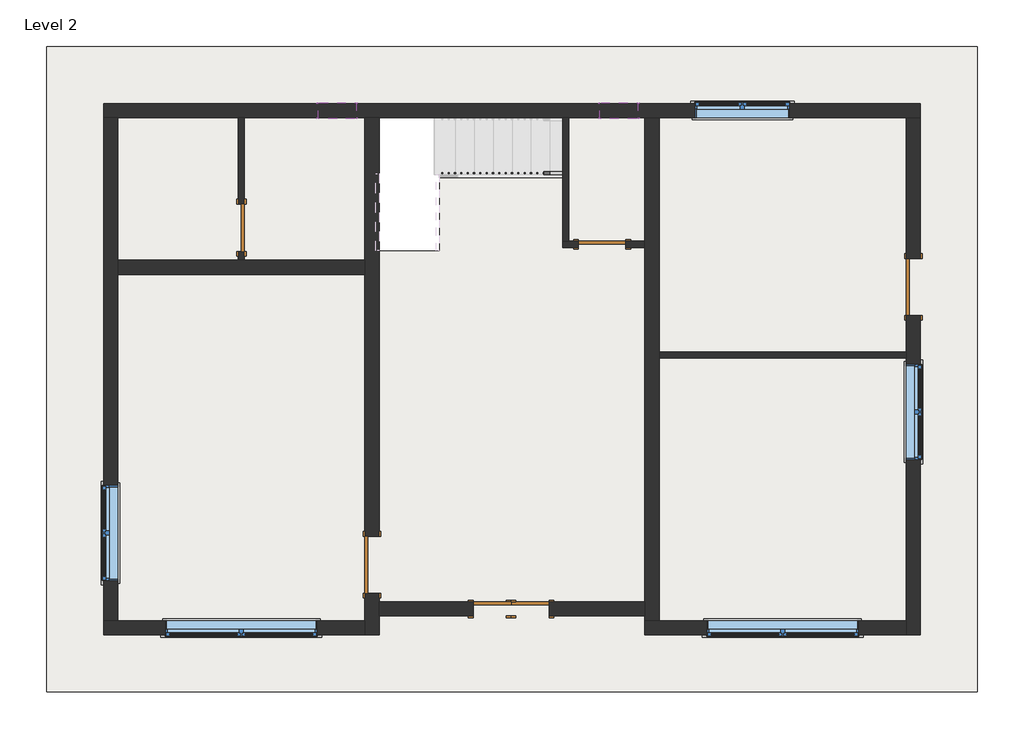
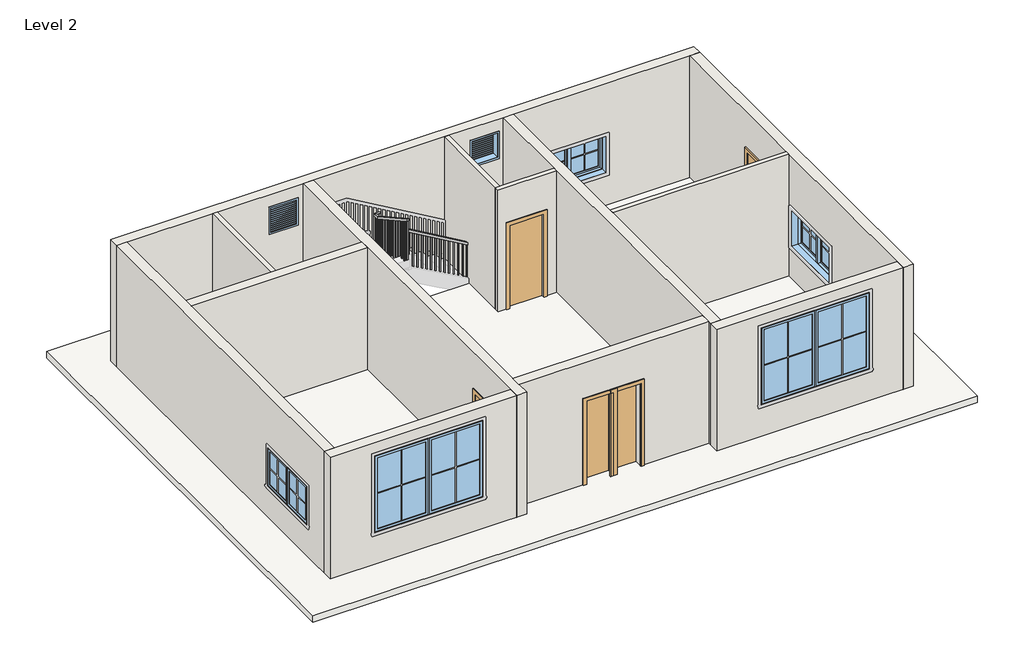
# One storey, part 1 of 2: 13 walls, 7 windows, 6 doors, 1 railing, 1 roof.
"""IFC4 building model written with IfcOpenShell, lengths in millimetres."""

from ifc_helpers import new_model, si_unit, frame, origin, place, context, project, spatial, polyline, outline, extrude, faceted_brep, transform, mapped, element, save
from components import single_flush_door_2_4a3212df, single_flush_door_2_0d3b4037, door_270f2424, door_aa9e95e7, single_flush_door_3_a90ba1ad, window_casement_double_c1d95f0f, window_casement_double_9ae172a2, window_f2d8fef0

model = new_model("IFC4")

# Units and contexts
model_context = context("Model", 3, world=origin())
ifc_project = project(units=[si_unit("LENGTHUNIT", "METRE", prefix="MILLI")], contexts=[model_context])

# Site, building, storey
site = spatial("IfcSite", under=ifc_project)
building = spatial("IfcBuilding", under=site)
storey = spatial("IfcBuildingStorey", under=building, Name="Level 2", Elevation=3048.0)

# Doors
placement = place(None, origin())
single_flush_door_2_shape = single_flush_door_2_4a3212df(model_context)
element("IfcDoor", 1, ObjectType="Single-Flush : DOOR 2'", at=placement, inside=storey, context=model_context, shape_type="MappedRepresentation", body=[
    mapped(single_flush_door_2_shape, transform((-1572.7415084, -2604.3618005, 3048.0), x_axis=(-1.0, 0.0, 0.0), y_axis=(0.0, -1.0, 0.0), z_axis=(0.0, 0.0, 1.0))),
])
single_flush_door_2_2_shape = single_flush_door_2_0d3b4037(model_context)
element("IfcDoor", 2, ObjectType="Single-Flush : DOOR 2'", at=placement, inside=storey, context=model_context, shape_type="MappedRepresentation", body=[
    mapped(single_flush_door_2_2_shape, transform((-963.1415084, -2604.3618005, 3048.0), x_axis=(1.0, 0.0, 0.0), y_axis=(0.0, 1.0, 0.0), z_axis=(0.0, 0.0, 1.0))),
])
door_shape = door_270f2424(model_context)
element("IfcDoor", 3, ObjectType="Single-Flush : DOOR 2'6\"", at=placement, inside=storey, context=model_context, shape_type="MappedRepresentation", body=[
    mapped(door_shape, transform((-5598.6415084, 3517.0381995, 3048.0), x_axis=(0.0, -1.0, 0.0), y_axis=(1.0, 0.0, 0.0), z_axis=(0.0, 0.0, 1.0))),
])
door_2_shape = door_aa9e95e7(model_context)
element("IfcDoor", 4, ObjectType="Single-Flush : DOOR 2'6\"", at=placement, inside=storey, context=model_context, shape_type="MappedRepresentation", body=[
    mapped(door_2_shape, transform((192.5584916, 3250.3381995, 3048.0), x_axis=(-1.0, 0.0, 0.0), y_axis=(0.0, -1.0, 0.0), z_axis=(0.0, 0.0, 1.0))),
])
single_flush_door_3_shape = single_flush_door_3_a90ba1ad(model_context)
element("IfcDoor", 5, ObjectType="Single-Flush : DOOR 3'", at=placement, inside=storey, context=model_context, shape_type="MappedRepresentation", body=[
    mapped(single_flush_door_3_shape, transform((-3503.1415084, -1893.1618005, 3048.0), x_axis=(0.0, -1.0, 0.0), y_axis=(1.0, 0.0, 0.0), z_axis=(0.0, 0.0, 1.0))),
])
element("IfcDoor", 6, ObjectType="Single-Flush : DOOR 3'", at=placement, inside=storey, context=model_context, shape_type="MappedRepresentation", body=[
    mapped(single_flush_door_3_shape, transform((5183.6584916, 2564.5381995, 3048.0), x_axis=(0.0, -1.0, 0.0), y_axis=(1.0, 0.0, 0.0), z_axis=(0.0, 0.0, 1.0))),
])

# Railing
element("IfcRailing", 7, ObjectType="Handrail - Rectangular", at=placement, inside=storey, context=model_context, shape_type="SolidModel", body=[
    faceted_brep([(-442.4415084, 4368.3146777, 4131.7333333), (-442.4415084, 4368.3146777, 4072.9219871), (-442.4415084, 4419.1146777, 4072.9219871), (-442.4415084, 4419.1146777, 4131.7333333), (-2398.2415084, 4368.3146777, 5272.6166667), (-2449.0415084, 4368.3146777, 5243.4386538), (-2449.0415084, 4419.1146777, 5243.4386538), (-2398.2415084, 4419.1146777, 5272.6166667), (-2398.2415084, 4368.3146777, 5528.7202697), (-2449.0415084, 4368.3146777, 5477.9202697), (-2449.0415084, 4419.1146777, 5477.9202697), (-2398.2415084, 4419.1146777, 5528.7202697), (-2474.4415084, 4368.3146777, 5528.7202697), (-2474.4415084, 4368.3146777, 5477.9202697), (-2525.2415084, 4419.1146777, 5477.9202697), (-2525.2415084, 4419.1146777, 5528.7202697), (-2474.4415084, 4292.1146777, 5528.7202697), (-2474.4415084, 4278.9546266, 5477.9202697), (-2525.2415084, 4278.9546266, 5477.9202697), (-2525.2415084, 4292.1146777, 5528.7202697), (-2474.4415084, 3148.7383287, 6163.7333333), (-2525.2415084, 3148.7383287, 6163.7333333), (-2525.2415084, 3148.7383287, 6105.62445), (-2474.4415084, 3148.7383287, 6105.62445)], [[[0, 1, 2, 3]], [[1, 0, 4, 5]], [[2, 1, 5, 6]], [[3, 2, 6, 7]], [[0, 3, 7, 4]], [[5, 4, 8, 9]], [[6, 5, 9, 10]], [[7, 6, 10, 11]], [[4, 7, 11, 8]], [[9, 8, 12, 13]], [[10, 9, 13, 14]], [[11, 10, 14, 15]], [[8, 11, 15, 12]], [[13, 12, 16, 17]], [[14, 13, 17, 18]], [[15, 14, 18, 19]], [[12, 15, 19, 16]], [[20, 21, 22, 23]], [[17, 16, 20, 23]], [[18, 17, 23, 22]], [[19, 18, 22, 21]], [[16, 19, 21, 20]]]),
    extrude(outline(polyline([(3184.0396777, 6086.1754052), (3184.0396777, 5080.0), (3164.9896777, 5080.0), (3164.9896777, 6096.7554726), (3184.0396777, 6086.1754052)])), frame((-2509.3665084, 0.0, 0.0), z_axis=(1.0, 0.0, 0.0), x_axis=(0.0, 1.0, 0.0)), (0.0, 0.0, 1.0), 19.05),
    extrude(outline(polyline([(3285.6396777, 6029.7483789), (3285.6396777, 5080.0), (3266.5896777, 5080.0), (3266.5896777, 6040.3284463), (3285.6396777, 6029.7483789)])), frame((-2509.3665084, 0.0, 0.0), z_axis=(1.0, 0.0, 0.0), x_axis=(0.0, 1.0, 0.0)), (0.0, 0.0, 1.0), 19.05),
    extrude(outline(polyline([(3387.2396777, 5973.3213526), (3387.2396777, 5080.0), (3368.1896777, 5080.0), (3368.1896777, 5983.9014201), (3387.2396777, 5973.3213526)])), frame((-2509.3665084, 0.0, 0.0), z_axis=(1.0, 0.0, 0.0), x_axis=(0.0, 1.0, 0.0)), (0.0, 0.0, 1.0), 19.05),
    extrude(outline(polyline([(3488.8396777, 5916.8420718), (3488.8396777, 4910.6666667), (3469.7896777, 4910.6666667), (3469.7896777, 5927.4221392), (3488.8396777, 5916.8420718)])), frame((-2509.3665084, 0.0, 0.0), z_axis=(1.0, 0.0, 0.0), x_axis=(0.0, 1.0, 0.0)), (0.0, 0.0, 1.0), 19.05),
    extrude(outline(polyline([(3590.4396777, 5860.4150456), (3590.4396777, 4910.6666667), (3571.3896777, 4910.6666667), (3571.3896777, 5870.995113), (3590.4396777, 5860.4150456)])), frame((-2509.3665084, 0.0, 0.0), z_axis=(1.0, 0.0, 0.0), x_axis=(0.0, 1.0, 0.0)), (0.0, 0.0, 1.0), 19.05),
    extrude(outline(polyline([(3692.0396777, 5803.9880193), (3692.0396777, 4910.6666667), (3672.9896777, 4910.6666667), (3672.9896777, 5814.5680867), (3692.0396777, 5803.9880193)])), frame((-2509.3665084, 0.0, 0.0), z_axis=(1.0, 0.0, 0.0), x_axis=(0.0, 1.0, 0.0)), (0.0, 0.0, 1.0), 19.05),
    extrude(outline(polyline([(3793.6396777, 5747.5087385), (3793.6396777, 4741.3333333), (3774.5896777, 4741.3333333), (3774.5896777, 5758.0888059), (3793.6396777, 5747.5087385)])), frame((-2509.3665084, 0.0, 0.0), z_axis=(1.0, 0.0, 0.0), x_axis=(0.0, 1.0, 0.0)), (0.0, 0.0, 1.0), 19.05),
    extrude(outline(polyline([(3895.2396777, 5691.0817122), (3895.2396777, 4741.3333333), (3876.1896777, 4741.3333333), (3876.1896777, 5701.6617797), (3895.2396777, 5691.0817122)])), frame((-2509.3665084, 0.0, 0.0), z_axis=(1.0, 0.0, 0.0), x_axis=(0.0, 1.0, 0.0)), (0.0, 0.0, 1.0), 19.05),
    extrude(outline(polyline([(3996.8396777, 5634.654686), (3996.8396777, 4741.3333333), (3977.7896777, 4741.3333333), (3977.7896777, 5645.2347534), (3996.8396777, 5634.654686)])), frame((-2509.3665084, 0.0, 0.0), z_axis=(1.0, 0.0, 0.0), x_axis=(0.0, 1.0, 0.0)), (0.0, 0.0, 1.0), 19.05),
    extrude(outline(polyline([(4098.4396777, 5578.1754052), (4098.4396777, 4572.0), (4079.3896777, 4572.0), (4079.3896777, 5588.7554726), (4098.4396777, 5578.1754052)])), frame((-2509.3665084, 0.0, 0.0), z_axis=(1.0, 0.0, 0.0), x_axis=(0.0, 1.0, 0.0)), (0.0, 0.0, 1.0), 19.05),
    extrude(outline(polyline([(4200.0396777, 5521.7483789), (4200.0396777, 4572.0), (4180.9896777, 4572.0), (4180.9896777, 5532.3284463), (4200.0396777, 5521.7483789)])), frame((-2509.3665084, 0.0, 0.0), z_axis=(1.0, 0.0, 0.0), x_axis=(0.0, 1.0, 0.0)), (0.0, 0.0, 1.0), 19.05),
    extrude(outline(polyline([(4301.6396777, 5465.3213526), (4301.6396777, 4572.0), (4282.5896777, 4572.0), (4282.5896777, 5475.9014201), (4301.6396777, 5465.3213526)])), frame((-2509.3665084, 0.0, 0.0), z_axis=(1.0, 0.0, 0.0), x_axis=(0.0, 1.0, 0.0)), (0.0, 0.0, 1.0), 19.05),
    extrude(outline(polyline([(-2464.9165084, 4384.1896777), (-2483.9665084, 4384.1896777), (-2483.9665084, 4403.2396777), (-2464.9165084, 4403.2396777), (-2464.9165084, 4384.1896777)])), frame((0.0, 0.0, 4402.6666667), z_axis=(0.0, 0.0, 1.0), x_axis=(1.0, 0.0, 0.0)), (0.0, 0.0, 1.0), 1075.253603),
    extrude(outline(polyline([(5204.5449038, -2382.3665084), (4233.3333333, -2382.3665084), (4233.3333333, -2363.3165084), (5193.4324038, -2363.3165084), (5204.5449038, -2382.3665084)])), frame((0.0, 4384.1896777, 0.0), z_axis=(0.0, 1.0, 0.0), x_axis=(0.0, 0.0, 1.0)), (0.0, 0.0, 1.0), 19.05),
    extrude(outline(polyline([(5145.2782371, -2280.7665084), (4233.3333333, -2280.7665084), (4233.3333333, -2261.7165084), (5134.1657371, -2261.7165084), (5145.2782371, -2280.7665084)])), frame((0.0, 4384.1896777, 0.0), z_axis=(0.0, 1.0, 0.0), x_axis=(0.0, 0.0, 1.0)), (0.0, 0.0, 1.0), 19.05),
    extrude(outline(polyline([(5086.0115704, -2179.1665084), (4233.3333333, -2179.1665084), (4233.3333333, -2160.1165084), (5074.8990704, -2160.1165084), (5086.0115704, -2179.1665084)])), frame((0.0, 4384.1896777, 0.0), z_axis=(0.0, 1.0, 0.0), x_axis=(0.0, 0.0, 1.0)), (0.0, 0.0, 1.0), 19.05),
    extrude(outline(polyline([(5026.7449038, -2077.5665084), (4064.0, -2077.5665084), (4064.0, -2058.5165084), (5015.6324038, -2058.5165084), (5026.7449038, -2077.5665084)])), frame((0.0, 4384.1896777, 0.0), z_axis=(0.0, 1.0, 0.0), x_axis=(0.0, 0.0, 1.0)), (0.0, 0.0, 1.0), 19.05),
    extrude(outline(polyline([(4967.4782371, -1975.9665084), (4064.0, -1975.9665084), (4064.0, -1956.9165084), (4956.3657371, -1956.9165084), (4967.4782371, -1975.9665084)])), frame((0.0, 4384.1896777, 0.0), z_axis=(0.0, 1.0, 0.0), x_axis=(0.0, 0.0, 1.0)), (0.0, 0.0, 1.0), 19.05),
    extrude(outline(polyline([(4908.2115704, -1874.3665084), (4064.0, -1874.3665084), (4064.0, -1855.3165084), (4897.0990704, -1855.3165084), (4908.2115704, -1874.3665084)])), frame((0.0, 4384.1896777, 0.0), z_axis=(0.0, 1.0, 0.0), x_axis=(0.0, 0.0, 1.0)), (0.0, 0.0, 1.0), 19.05),
    extrude(outline(polyline([(4848.9449038, -1772.7665084), (3894.6666667, -1772.7665084), (3894.6666667, -1753.7165084), (4837.8324038, -1753.7165084), (4848.9449038, -1772.7665084)])), frame((0.0, 4384.1896777, 0.0), z_axis=(0.0, 1.0, 0.0), x_axis=(0.0, 0.0, 1.0)), (0.0, 0.0, 1.0), 19.05),
    extrude(outline(polyline([(4789.6782371, -1671.1665084), (3894.6666667, -1671.1665084), (3894.6666667, -1652.1165084), (4778.5657371, -1652.1165084), (4789.6782371, -1671.1665084)])), frame((0.0, 4384.1896777, 0.0), z_axis=(0.0, 1.0, 0.0), x_axis=(0.0, 0.0, 1.0)), (0.0, 0.0, 1.0), 19.05),
    extrude(outline(polyline([(4730.4115704, -1569.5665084), (3894.6666667, -1569.5665084), (3894.6666667, -1550.5165084), (4719.2990704, -1550.5165084), (4730.4115704, -1569.5665084)])), frame((0.0, 4384.1896777, 0.0), z_axis=(0.0, 1.0, 0.0), x_axis=(0.0, 0.0, 1.0)), (0.0, 0.0, 1.0), 19.05),
    extrude(outline(polyline([(4671.1449038, -1467.9665084), (3725.3333333, -1467.9665084), (3725.3333333, -1448.9165084), (4660.0324038, -1448.9165084), (4671.1449038, -1467.9665084)])), frame((0.0, 4384.1896777, 0.0), z_axis=(0.0, 1.0, 0.0), x_axis=(0.0, 0.0, 1.0)), (0.0, 0.0, 1.0), 19.05),
    extrude(outline(polyline([(4611.8782371, -1366.3665084), (3725.3333333, -1366.3665084), (3725.3333333, -1347.3165084), (4600.7657371, -1347.3165084), (4611.8782371, -1366.3665084)])), frame((0.0, 4384.1896777, 0.0), z_axis=(0.0, 1.0, 0.0), x_axis=(0.0, 0.0, 1.0)), (0.0, 0.0, 1.0), 19.05),
    extrude(outline(polyline([(4552.6115704, -1264.7665084), (3725.3333333, -1264.7665084), (3725.3333333, -1245.7165084), (4541.4990704, -1245.7165084), (4552.6115704, -1264.7665084)])), frame((0.0, 4384.1896777, 0.0), z_axis=(0.0, 1.0, 0.0), x_axis=(0.0, 0.0, 1.0)), (0.0, 0.0, 1.0), 19.05),
    extrude(outline(polyline([(4493.3449038, -1163.1665084), (3556.0, -1163.1665084), (3556.0, -1144.1165084), (4482.2324038, -1144.1165084), (4493.3449038, -1163.1665084)])), frame((0.0, 4384.1896777, 0.0), z_axis=(0.0, 1.0, 0.0), x_axis=(0.0, 0.0, 1.0)), (0.0, 0.0, 1.0), 19.05),
    extrude(outline(polyline([(4434.0782371, -1061.5665084), (3556.0, -1061.5665084), (3556.0, -1042.5165084), (4422.9657371, -1042.5165084), (4434.0782371, -1061.5665084)])), frame((0.0, 4384.1896777, 0.0), z_axis=(0.0, 1.0, 0.0), x_axis=(0.0, 0.0, 1.0)), (0.0, 0.0, 1.0), 19.05),
    extrude(outline(polyline([(4374.8115704, -959.9665084), (3556.0, -959.9665084), (3556.0, -940.9165084), (4363.6990704, -940.9165084), (4374.8115704, -959.9665084)])), frame((0.0, 4384.1896777, 0.0), z_axis=(0.0, 1.0, 0.0), x_axis=(0.0, 0.0, 1.0)), (0.0, 0.0, 1.0), 19.05),
    extrude(outline(polyline([(4315.5449038, -858.3665084), (3386.6666667, -858.3665084), (3386.6666667, -839.3165084), (4304.4324038, -839.3165084), (4315.5449038, -858.3665084)])), frame((0.0, 4384.1896777, 0.0), z_axis=(0.0, 1.0, 0.0), x_axis=(0.0, 0.0, 1.0)), (0.0, 0.0, 1.0), 19.05),
    extrude(outline(polyline([(4256.2782371, -756.7665084), (3386.6666667, -756.7665084), (3386.6666667, -737.7165084), (4245.1657371, -737.7165084), (4256.2782371, -756.7665084)])), frame((0.0, 4384.1896777, 0.0), z_axis=(0.0, 1.0, 0.0), x_axis=(0.0, 0.0, 1.0)), (0.0, 0.0, 1.0), 19.05),
    extrude(outline(polyline([(4197.0115704, -655.1665084), (3386.6666667, -655.1665084), (3386.6666667, -636.1165084), (4185.8990704, -636.1165084), (4197.0115704, -655.1665084)])), frame((0.0, 4384.1896777, 0.0), z_axis=(0.0, 1.0, 0.0), x_axis=(0.0, 0.0, 1.0)), (0.0, 0.0, 1.0), 19.05),
    extrude(outline(polyline([(4137.7449038, -553.5665084), (3217.3333333, -553.5665084), (3217.3333333, -534.5165084), (4126.6324038, -534.5165084), (4137.7449038, -553.5665084)])), frame((0.0, 4384.1896777, 0.0), z_axis=(0.0, 1.0, 0.0), x_axis=(0.0, 0.0, 1.0)), (0.0, 0.0, 1.0), 19.05),
    extrude(outline(polyline([(-2490.3165084, 4384.1896777), (-2509.3665084, 4384.1896777), (-2509.3665084, 4403.2396777), (-2490.3165084, 4403.2396777), (-2490.3165084, 4384.1896777)])), frame((0.0, 0.0, 4402.6666667), z_axis=(0.0, 0.0, 1.0), x_axis=(1.0, 0.0, 0.0)), (0.0, 0.0, 1.0), 1075.253603),
    extrude(outline(polyline([(3167.7883287, 6095.0443826), (3167.7883287, 5080.0), (3148.7383287, 5080.0), (3148.7383287, 6105.62445), (3167.7883287, 6095.0443826)])), frame((-2509.3665084, 0.0, 0.0), z_axis=(1.0, 0.0, 0.0), x_axis=(0.0, 1.0, 0.0)), (0.0, 0.0, 1.0), 19.05),
    extrude(outline(polyline([(4084.0344871, -461.4915084), (3217.3333333, -461.4915084), (3217.3333333, -442.4415084), (4072.9219871, -442.4415084), (4084.0344871, -461.4915084)])), frame((0.0, 4384.1896777, 0.0), z_axis=(0.0, 1.0, 0.0), x_axis=(0.0, 0.0, 1.0)), (0.0, 0.0, 1.0), 19.05),
])

# Roof
element("IfcRoof", 8, ObjectType="ROOF 6\"", at=placement, inside=storey, context=model_context, shape_type="SweptSolid", body=[
    extrude(outline(polyline([(-8722.8415084, -3937.8618005), (-8722.8415084, 6425.3381995), (6212.3584916, 6425.3381995), (6212.3584916, -3937.8618005), (-8722.8415084, -3937.8618005)]), holes=[polyline([(-3439.6415084, 5333.1381995), (-3439.6415084, 3148.7383287), (-2423.6415084, 3148.7383287), (-2423.6415084, 4317.5146777), (-442.4415084, 4317.5146777), (-442.4415084, 5333.1381995), (-3439.6415084, 5333.1381995)])]), frame((0.0, 0.0, 3048.0), z_axis=(0.0, 0.0, 1.0), x_axis=(1.0, 0.0, 0.0)), (0.0, 0.0, 1.0), 152.4),
])

# Walls
element("IfcWall", 9, ObjectType="WALL 4\"", at=placement, inside=storey, context=model_context, shape_type="SweptSolid", body=[
    extrude(outline(polyline([(3136.0381995, 5181.6), (3136.0381995, 3048.0), (2996.3381995, 3048.0), (2996.3381995, 6096.0), (5282.3381995, 6096.0), (5282.3381995, 3048.0), (3898.0381995, 3048.0), (3898.0381995, 5181.6), (3136.0381995, 5181.6)])), frame((-5649.4415084, 0.0, 0.0), z_axis=(1.0, 0.0, 0.0), x_axis=(0.0, 1.0, 0.0)), (0.0, 0.0, 1.0), 101.6),
])
element("IfcWall", 10, ObjectType="WALL 4\"", at=placement, inside=storey, context=model_context, shape_type="Brep", body=[
    faceted_brep([(-188.4415084, 3301.1381995, 5181.6), (-188.4415084, 3301.1381995, 3048.0), (-340.8415084, 3301.1381995, 3048.0), (-442.4415084, 3301.1381995, 3048.0), (-442.4415084, 3301.1381995, 6096.0), (-340.8415084, 3301.1381995, 6096.0), (878.3584916, 3301.1381995, 6096.0), (878.3584916, 3301.1381995, 3048.0), (573.5584916, 3301.1381995, 3048.0), (573.5584916, 3301.1381995, 5181.6), (-442.4415084, 3199.5381995, 3048.0), (-188.4415084, 3199.5381995, 3048.0), (-188.4415084, 3199.5381995, 5181.6), (573.5584916, 3199.5381995, 5181.6), (573.5584916, 3199.5381995, 3048.0), (878.3584916, 3199.5381995, 3048.0), (878.3584916, 3199.5381995, 6096.0), (-442.4415084, 3199.5381995, 6096.0)], [[[0, 1, 2, 3, 4, 5, 6, 7, 8, 9]], [[10, 11, 12, 13, 14, 15, 16, 17]], [[8, 7, 15, 14]], [[3, 2, 1, 11, 10]], [[7, 6, 16, 15]], [[4, 3, 10, 17]], [[12, 11, 1, 0]], [[13, 12, 0, 9]], [[14, 13, 9, 8]], [[6, 5, 4, 17, 16]]]),
])
element("IfcWall", 11, ObjectType="WALL 4\"", at=placement, inside=storey, context=model_context, shape_type="Brep", body=[
    faceted_brep([(-340.8415084, 3301.1381995, 3048.0), (-340.8415084, 5282.3381995, 3048.0), (-340.8415084, 5282.3381995, 6096.0), (-340.8415084, 3301.1381995, 6096.0), (-442.4415084, 3301.1381995, 3048.0), (-442.4415084, 3301.1381995, 6096.0), (-442.4415084, 4317.5146777, 6096.0), (-442.4415084, 5282.3381995, 6096.0), (-442.4415084, 5282.3381995, 3048.0)], [[[0, 1, 2, 3]], [[4, 5, 6, 7, 8]], [[1, 0, 4, 8]], [[0, 3, 5, 4]], [[2, 1, 8, 7]], [[3, 2, 7, 6, 5]]]),
])
element("IfcWall", 12, ObjectType="WALL 4\"", at=placement, inside=storey, context=model_context, shape_type="SweptSolid", body=[
    extrude(outline(polyline([(1106.9584916, 1523.1381995), (5069.3584916, 1523.1381995), (5069.3584916, 1421.5381995), (1106.9584916, 1421.5381995), (1106.9584916, 1523.1381995)])), frame((0.0, 0.0, 3048.0), z_axis=(0.0, 0.0, 1.0), x_axis=(1.0, 0.0, 0.0)), (0.0, 0.0, 1.0), 3048.0),
])
element("IfcWall", 13, ObjectType="WALL 9\"", at=placement, inside=storey, context=model_context, shape_type="Brep", body=[
    faceted_brep([(-7808.4415084, 5282.3381995, 3048.0), (-7579.8415084, 5282.3381995, 3048.0), (-5649.4415084, 5282.3381995, 3048.0), (-5547.8415084, 5282.3381995, 3048.0), (-3617.4415084, 5282.3381995, 3048.0), (-3388.8415084, 5282.3381995, 3048.0), (-442.4415084, 5282.3381995, 3048.0), (-340.8415084, 5282.3381995, 3048.0), (878.3584916, 5282.3381995, 3048.0), (1106.9584916, 5282.3381995, 3048.0), (5069.3584916, 5282.3381995, 3048.0), (5297.9584916, 5282.3381995, 3048.0), (5297.9584916, 5282.3381995, 6096.0), (5069.3584916, 5282.3381995, 6096.0), (1106.9584916, 5282.3381995, 6096.0), (878.3584916, 5282.3381995, 6096.0), (-340.8415084, 5282.3381995, 6096.0), (-442.4415084, 5282.3381995, 6096.0), (-3388.8415084, 5282.3381995, 6096.0), (-3617.4415084, 5282.3381995, 6096.0), (-5547.8415084, 5282.3381995, 6096.0), (-5649.4415084, 5282.3381995, 6096.0), (-7579.8415084, 5282.3381995, 6096.0), (-7808.4415084, 5282.3381995, 6096.0), (3202.4584916, 5282.3381995, 4876.8), (3202.4584916, 5282.3381995, 3962.4), (1678.4584916, 5282.3381995, 3962.4), (1678.4584916, 5282.3381995, 4876.8), (154.4584916, 5282.3381995, 5791.2), (764.0584916, 5282.3381995, 5791.2), (764.0584916, 5282.3381995, 5181.6), (154.4584916, 5282.3381995, 5181.6), (-3757.1415084, 5282.3381995, 5791.2), (-3757.1415084, 5282.3381995, 5181.6), (-4366.7415084, 5282.3381995, 5181.6), (-4366.7415084, 5282.3381995, 5791.2), (-7808.4415084, 5510.9381995, 3048.0), (-7808.4415084, 5510.9381995, 6096.0), (5297.9584916, 5510.9381995, 6096.0), (5297.9584916, 5510.9381995, 3048.0), (3202.4584916, 5510.9381995, 4876.8), (1678.4584916, 5510.9381995, 4876.8), (1678.4584916, 5510.9381995, 3962.4), (3202.4584916, 5510.9381995, 3962.4), (154.4584916, 5510.9381995, 5791.2), (154.4584916, 5510.9381995, 5181.6), (764.0584916, 5510.9381995, 5181.6), (764.0584916, 5510.9381995, 5791.2), (-3757.1415084, 5510.9381995, 5791.2), (-4366.7415084, 5510.9381995, 5791.2), (-4366.7415084, 5510.9381995, 5181.6), (-3757.1415084, 5510.9381995, 5181.6)], [[[0, 1, 2, 3, 4, 5, 6, 7, 8, 9, 10, 11, 12, 13, 14, 15, 16, 17, 18, 19, 20, 21, 22, 23], [24, 25, 26, 27], [28, 29, 30, 31], [32, 33, 34, 35]], [[36, 37, 38, 39], [40, 41, 42, 43], [44, 45, 46, 47], [48, 49, 50, 51]], [[11, 10, 9, 8, 7, 6, 5, 4, 3, 2, 1, 0, 36, 39]], [[23, 22, 21, 20, 19, 18, 17, 16, 15, 14, 13, 12, 38, 37]], [[12, 11, 39, 38]], [[0, 23, 37, 36]], [[25, 24, 40, 43]], [[26, 25, 43, 42]], [[27, 26, 42, 41]], [[24, 27, 41, 40]], [[45, 44, 28, 31]], [[46, 45, 31, 30]], [[47, 46, 30, 29]], [[44, 47, 29, 28]], [[33, 32, 48, 51]], [[34, 33, 51, 50]], [[35, 34, 50, 49]], [[32, 35, 49, 48]]]),
])
element("IfcWall", 14, ObjectType="WALL 9\"", at=placement, inside=storey, context=model_context, shape_type="Brep", body=[
    faceted_brep([(5069.3584916, 2107.3381995, 5181.6), (5069.3584916, 2107.3381995, 3048.0), (5069.3584916, 1523.1381995, 3048.0), (5069.3584916, 1421.5381995, 3048.0), (5069.3584916, -2794.8618005, 3048.0), (5069.3584916, -3023.4618005, 3048.0), (5069.3584916, -3023.4618005, 6096.0), (5069.3584916, -2794.8618005, 6096.0), (5069.3584916, 1421.5381995, 6096.0), (5069.3584916, 1523.1381995, 6096.0), (5069.3584916, 5282.3381995, 6096.0), (5069.3584916, 5282.3381995, 3048.0), (5069.3584916, 3021.7381995, 3048.0), (5069.3584916, 3021.7381995, 5181.6), (5069.3584916, -204.0618005, 4876.8), (5069.3584916, -204.0618005, 3962.4), (5069.3584916, 1319.9381995, 3962.4), (5069.3584916, 1319.9381995, 4876.8), (5297.9584916, -3023.4618005, 3048.0), (5297.9584916, 2107.3381995, 3048.0), (5297.9584916, 2107.3381995, 5181.6), (5297.9584916, 3021.7381995, 5181.6), (5297.9584916, 3021.7381995, 3048.0), (5297.9584916, 5282.3381995, 3048.0), (5297.9584916, 5282.3381995, 6096.0), (5297.9584916, -3023.4618005, 6096.0), (5297.9584916, -204.0618005, 4876.8), (5297.9584916, 1319.9381995, 4876.8), (5297.9584916, 1319.9381995, 3962.4), (5297.9584916, -204.0618005, 3962.4)], [[[0, 1, 2, 3, 4, 5, 6, 7, 8, 9, 10, 11, 12, 13], [14, 15, 16, 17]], [[18, 19, 20, 21, 22, 23, 24, 25], [26, 27, 28, 29]], [[12, 11, 23, 22]], [[5, 4, 3, 2, 1, 19, 18]], [[11, 10, 24, 23]], [[6, 5, 18, 25]], [[15, 14, 26, 29]], [[16, 15, 29, 28]], [[17, 16, 28, 27]], [[14, 17, 27, 26]], [[20, 19, 1, 0]], [[21, 20, 0, 13]], [[22, 21, 13, 12]], [[10, 9, 8, 7, 6, 25, 24]]]),
])
element("IfcWall", 15, ObjectType="WALL 9\"", at=placement, inside=storey, context=model_context, shape_type="Brep", body=[
    faceted_brep([(5069.3584916, -2794.8618005, 3048.0), (1106.9584916, -2794.8618005, 3048.0), (878.3584916, -2794.8618005, 3048.0), (878.3584916, -2794.8618005, 6096.0), (1106.9584916, -2794.8618005, 6096.0), (5069.3584916, -2794.8618005, 6096.0), (1868.9584916, -2794.8618005, 5791.2), (1868.9584916, -2794.8618005, 3962.4), (4307.3584916, -2794.8618005, 3962.4), (4307.3584916, -2794.8618005, 5791.2), (5069.3584916, -3023.4618005, 3048.0), (5069.3584916, -3023.4618005, 6096.0), (878.3584916, -3023.4618005, 6096.0), (878.3584916, -3023.4618005, 3048.0), (1868.9584916, -3023.4618005, 5791.2), (4307.3584916, -3023.4618005, 5791.2), (4307.3584916, -3023.4618005, 3962.4), (1868.9584916, -3023.4618005, 3962.4)], [[[0, 1, 2, 3, 4, 5], [6, 7, 8, 9]], [[10, 11, 12, 13], [14, 15, 16, 17]], [[2, 1, 0, 10, 13]], [[0, 5, 11, 10]], [[3, 2, 13, 12]], [[7, 6, 14, 17]], [[8, 7, 17, 16]], [[9, 8, 16, 15]], [[6, 9, 15, 14]], [[5, 4, 3, 12, 11]]]),
])
element("IfcWall", 16, ObjectType="WALL 9\"", at=placement, inside=storey, context=model_context, shape_type="Brep", body=[
    faceted_brep([(1106.9584916, -2794.8618005, 3048.0), (1106.9584916, 1421.5381995, 3048.0), (1106.9584916, 1523.1381995, 3048.0), (1106.9584916, 5282.3381995, 3048.0), (1106.9584916, 5282.3381995, 6096.0), (1106.9584916, 1523.1381995, 6096.0), (1106.9584916, 1421.5381995, 6096.0), (1106.9584916, -2794.8618005, 6096.0), (878.3584916, -2794.8618005, 3048.0), (878.3584916, -2794.8618005, 6096.0), (878.3584916, -2718.6618005, 6096.0), (878.3584916, -2490.0618005, 6096.0), (878.3584916, 3199.5381995, 6096.0), (878.3584916, 3301.1381995, 6096.0), (878.3584916, 5282.3381995, 6096.0), (878.3584916, 5282.3381995, 3048.0), (878.3584916, 3301.1381995, 3048.0), (878.3584916, 3199.5381995, 3048.0), (878.3584916, -2490.0618005, 3048.0), (878.3584916, -2718.6618005, 3048.0)], [[[0, 1, 2, 3, 4, 5, 6, 7]], [[8, 9, 10, 11, 12, 13, 14, 15, 16, 17, 18, 19]], [[3, 2, 1, 0, 8, 19, 18, 17, 16, 15]], [[0, 7, 9, 8]], [[4, 3, 15, 14]], [[7, 6, 5, 4, 14, 13, 12, 11, 10, 9]]]),
])
element("IfcWall", 17, ObjectType="WALL 9\"", at=placement, inside=storey, context=model_context, shape_type="SweptSolid", body=[
    extrude(outline(polyline([(3048.0, 878.3584916), (6096.0, 878.3584916), (6096.0, -3388.8415084), (3048.0, -3388.8415084), (3048.0, -1877.5415084), (5181.6, -1877.5415084), (5181.6, -658.3415084), (3048.0, -658.3415084), (3048.0, 878.3584916)])), frame((0.0, -2718.6618005, 0.0), z_axis=(0.0, 1.0, 0.0), x_axis=(0.0, 0.0, 1.0)), (0.0, 0.0, 1.0), 228.6),
])
element("IfcWall", 18, ObjectType="WALL 9\"", at=placement, inside=storey, context=model_context, shape_type="Brep", body=[
    faceted_brep([(-3388.8415084, -3023.4618005, 3048.0), (-3388.8415084, -2718.6618005, 3048.0), (-3388.8415084, -2490.0618005, 3048.0), (-3388.8415084, -2350.3618005, 3048.0), (-3388.8415084, -2350.3618005, 5181.6), (-3388.8415084, -1435.9618005, 5181.6), (-3388.8415084, -1435.9618005, 3048.0), (-3388.8415084, 5282.3381995, 3048.0), (-3388.8415084, 5282.3381995, 6096.0), (-3388.8415084, -2490.0618005, 6096.0), (-3388.8415084, -2718.6618005, 6096.0), (-3388.8415084, -3023.4618005, 6096.0), (-3617.4415084, -2350.3618005, 5181.6), (-3617.4415084, -2350.3618005, 3048.0), (-3617.4415084, -2794.8618005, 3048.0), (-3617.4415084, -3023.4618005, 3048.0), (-3617.4415084, -3023.4618005, 6096.0), (-3617.4415084, -2794.8618005, 6096.0), (-3617.4415084, 2767.7381995, 6096.0), (-3617.4415084, 2996.3381995, 6096.0), (-3617.4415084, 5282.3381995, 6096.0), (-3617.4415084, 5282.3381995, 3048.0), (-3617.4415084, 2996.3381995, 3048.0), (-3617.4415084, 2767.7381995, 3048.0), (-3617.4415084, -1435.9618005, 3048.0), (-3617.4415084, -1435.9618005, 5181.6)], [[[0, 1, 2, 3, 4, 5, 6, 7, 8, 9, 10, 11]], [[12, 13, 14, 15, 16, 17, 18, 19, 20, 21, 22, 23, 24, 25]], [[15, 14, 13, 3, 2, 1, 0]], [[24, 23, 22, 21, 7, 6]], [[11, 10, 9, 8, 20, 19, 18, 17, 16]], [[8, 7, 21, 20]], [[0, 11, 16, 15]], [[4, 3, 13, 12]], [[5, 4, 12, 25]], [[6, 5, 25, 24]]]),
])
element("IfcWall", 19, ObjectType="WALL 9\"", at=placement, inside=storey, context=model_context, shape_type="Brep", body=[
    faceted_brep([(-3617.4415084, -2794.8618005, 3048.0), (-7579.8415084, -2794.8618005, 3048.0), (-7808.4415084, -2794.8618005, 3048.0), (-7808.4415084, -2794.8618005, 6096.0), (-7579.8415084, -2794.8618005, 6096.0), (-3617.4415084, -2794.8618005, 6096.0), (-6817.8415084, -2794.8618005, 5791.2), (-6817.8415084, -2794.8618005, 3962.4), (-4379.4415084, -2794.8618005, 3962.4), (-4379.4415084, -2794.8618005, 5791.2), (-3617.4415084, -3023.4618005, 3048.0), (-3617.4415084, -3023.4618005, 6096.0), (-7808.4415084, -3023.4618005, 6096.0), (-7808.4415084, -3023.4618005, 3048.0), (-6817.8415084, -3023.4618005, 5791.2), (-4379.4415084, -3023.4618005, 5791.2), (-4379.4415084, -3023.4618005, 3962.4), (-6817.8415084, -3023.4618005, 3962.4)], [[[0, 1, 2, 3, 4, 5], [6, 7, 8, 9]], [[10, 11, 12, 13], [14, 15, 16, 17]], [[2, 1, 0, 10, 13]], [[0, 5, 11, 10]], [[3, 2, 13, 12]], [[7, 6, 14, 17]], [[8, 7, 17, 16]], [[9, 8, 16, 15]], [[6, 9, 15, 14]], [[5, 4, 3, 12, 11]]]),
])
element("IfcWall", 20, ObjectType="WALL 9\"", at=placement, inside=storey, context=model_context, shape_type="Brep", body=[
    faceted_brep([(-7579.8415084, -2794.8618005, 3048.0), (-7579.8415084, 2767.7381995, 3048.0), (-7579.8415084, 2996.3381995, 3048.0), (-7579.8415084, 5282.3381995, 3048.0), (-7579.8415084, 5282.3381995, 6096.0), (-7579.8415084, 2996.3381995, 6096.0), (-7579.8415084, 2767.7381995, 6096.0), (-7579.8415084, -2794.8618005, 6096.0), (-7579.8415084, -623.1618005, 4876.8), (-7579.8415084, -623.1618005, 3962.4), (-7579.8415084, -2147.1618005, 3962.4), (-7579.8415084, -2147.1618005, 4876.8), (-7808.4415084, -2794.8618005, 3048.0), (-7808.4415084, -2794.8618005, 6096.0), (-7808.4415084, 5282.3381995, 6096.0), (-7808.4415084, 5282.3381995, 3048.0), (-7808.4415084, -623.1618005, 4876.8), (-7808.4415084, -2147.1618005, 4876.8), (-7808.4415084, -2147.1618005, 3962.4), (-7808.4415084, -623.1618005, 3962.4)], [[[0, 1, 2, 3, 4, 5, 6, 7], [8, 9, 10, 11]], [[12, 13, 14, 15], [16, 17, 18, 19]], [[3, 2, 1, 0, 12, 15]], [[0, 7, 13, 12]], [[4, 3, 15, 14]], [[9, 8, 16, 19]], [[10, 9, 19, 18]], [[11, 10, 18, 17]], [[8, 11, 17, 16]], [[7, 6, 5, 4, 14, 13]]]),
])
element("IfcWall", 21, ObjectType="WALL 9\"", at=placement, inside=storey, context=model_context, shape_type="Brep", body=[
    faceted_brep([(-7579.8415084, 2767.7381995, 3048.0), (-3617.4415084, 2767.7381995, 3048.0), (-3617.4415084, 2767.7381995, 6096.0), (-7579.8415084, 2767.7381995, 6096.0), (-7579.8415084, 2996.3381995, 3048.0), (-7579.8415084, 2996.3381995, 6096.0), (-5649.4415084, 2996.3381995, 6096.0), (-5547.8415084, 2996.3381995, 6096.0), (-3617.4415084, 2996.3381995, 6096.0), (-3617.4415084, 2996.3381995, 3048.0), (-5547.8415084, 2996.3381995, 3048.0), (-5649.4415084, 2996.3381995, 3048.0)], [[[0, 1, 2, 3]], [[4, 5, 6, 7, 8, 9, 10, 11]], [[1, 0, 4, 11, 10, 9]], [[2, 1, 9, 8]], [[0, 3, 5, 4]], [[3, 2, 8, 7, 6, 5]]]),
])

# Windows
window_casement_double_shape = window_casement_double_c1d95f0f(model_context)
element("IfcWindow", 22, ObjectType="Window-Casement-Double", at=placement, inside=storey, context=model_context, shape_type="MappedRepresentation", body=[
    mapped(window_casement_double_shape, transform((-7694.1415084, -1385.1618005, 3048.0), x_axis=(0.0, 1.0, 0.0), y_axis=(-1.0, 0.0, 0.0), z_axis=(0.0, 0.0, 1.0))),
])
element("IfcWindow", 23, ObjectType="Window-Casement-Double", at=placement, inside=storey, context=model_context, shape_type="MappedRepresentation", body=[
    mapped(window_casement_double_shape, transform((5183.6584916, 557.9381995, 3048.0), x_axis=(0.0, -1.0, 0.0), y_axis=(1.0, 0.0, 0.0), z_axis=(0.0, 0.0, 1.0))),
])
element("IfcWindow", 24, ObjectType="Window-Casement-Double", at=placement, inside=storey, context=model_context, shape_type="MappedRepresentation", body=[
    mapped(window_casement_double_shape, transform((2440.4584916, 5396.6381995, 3048.0), x_axis=(1.0, 0.0, 0.0), y_axis=(0.0, 1.0, 0.0), z_axis=(0.0, 0.0, 1.0))),
])
window_casement_double_2_shape = window_casement_double_9ae172a2(model_context)
element("IfcWindow", 25, ObjectType="Window-Casement-Double", at=placement, inside=storey, context=model_context, shape_type="MappedRepresentation", body=[
    mapped(window_casement_double_2_shape, transform((-5598.6415084, -2909.1618005, 3048.0), x_axis=(-1.0, 0.0, 0.0), y_axis=(0.0, -1.0, 0.0), z_axis=(0.0, 0.0, 1.0))),
])
element("IfcWindow", 26, ObjectType="Window-Casement-Double", at=placement, inside=storey, context=model_context, shape_type="MappedRepresentation", body=[
    mapped(window_casement_double_2_shape, transform((3088.1584916, -2909.1618005, 3048.0), x_axis=(-1.0, 0.0, 0.0), y_axis=(0.0, -1.0, 0.0), z_axis=(0.0, 0.0, 1.0))),
])
window_shape = window_f2d8fef0(model_context)
element("IfcWindow", 27, ObjectType="Window-Louvers : 24\" x 24\"", at=placement, inside=storey, context=model_context, shape_type="MappedRepresentation", body=[
    mapped(window_shape, transform((459.2584916, 5402.9881995, 4267.2), x_axis=(1.0, 0.0, 0.0), y_axis=(0.0, 1.0, 0.0), z_axis=(0.0, 0.0, 1.0))),
])
element("IfcWindow", 28, ObjectType="Window-Louvers : 24\" x 24\"", at=placement, inside=storey, context=model_context, shape_type="MappedRepresentation", body=[
    mapped(window_shape, transform((-4061.9415084, 5390.2881995, 4267.2), x_axis=(-1.0, 0.0, 0.0), y_axis=(0.0, -1.0, 0.0), z_axis=(0.0, 0.0, 1.0))),
])

save(model, "model.ifc")

# Revit data of these elements
# Type "Single-Flush : DOOR 2'"
#   Type Mark = "10"
#   Construction Type Id = "MDOOR"
#   Assembly Code = "C1020"
#   Analytic Construction = "Metal"
#   Thickness = 0' - 2"
#   Heat Transfer Coefficient (U) = 0.651978 BTU/(h·ft²·°F)
#   Height = 7' - 0"
#   Trim Projection Ext = 0' - 1"
#   Trim Projection Int = 0' - 1"
#   Trim Width = 0' - 3"
#   Width = 2' - 0"
#   Define Thermal Properties by = 1
#   Door Material = Door - Panel
#   Frame Material = Door - Frame
#   Visual Light Transmittance = 0
#   Solar Heat Gain Coefficient = 0
#   Function = (empty or 0)
#   Wall Closure = (empty or 0)
# Type "Single-Flush : DOOR 2'6\""
#   Type Mark = "9"
#   Construction Type Id = "MDOOR"
#   Assembly Code = "C1020"
#   Analytic Construction = "Metal"
#   Thickness = 0' - 2"
#   Heat Transfer Coefficient (U) = 0.651978 BTU/(h·ft²·°F)
#   Height = 7' - 0"
#   Trim Projection Ext = 0' - 1"
#   Trim Projection Int = 0' - 1"
#   Trim Width = 0' - 3"
#   Width = 2' - 6"
#   Define Thermal Properties by = 1
#   Door Material = Door - Panel
#   Frame Material = Door - Frame
#   Visual Light Transmittance = 0
#   Solar Heat Gain Coefficient = 0
#   Function = (empty or 0)
#   Wall Closure = (empty or 0)
# Type "Single-Flush : DOOR 3'"
#   Type Mark = "8"
#   Construction Type Id = "MDOOR"
#   Assembly Code = "C1020"
#   Analytic Construction = "Metal"
#   Thickness = 0' - 2"
#   Heat Transfer Coefficient (U) = 0.651978 BTU/(h·ft²·°F)
#   Height = 7' - 0"
#   Trim Projection Ext = 0' - 1"
#   Trim Projection Int = 0' - 1"
#   Trim Width = 0' - 3"
#   Width = 3' - 0"
#   Define Thermal Properties by = 1
#   Door Material = Door - Panel
#   Frame Material = Door - Frame
#   Visual Light Transmittance = 0
#   Solar Heat Gain Coefficient = 0
#   Function = (empty or 0)
#   Wall Closure = (empty or 0)
# Type "Handrail - Rectangular"
#   Assembly Code = "C2010400"
#   built-in parameter 1008612 = 0.0416667 (stored number, unit not read)
#   built-in parameter 1008611 = 0.0416667 (stored number, unit not read)
#   built-in parameter 1008609 = 0.333333 (stored number, unit not read)
#   built-in parameter 1008604 = 0.166667 (stored number, unit not read)
#   built-in parameter 1008603 = 0.166667 (stored number, unit not read)
#   Railing Height = 3' - 0"
#   built-in parameter 1008630 = 2
#   built-in parameter 1008610 = 2
#   built-in parameter 1008618 = Baluster - Square : 3/4"
# Type "ROOF 6\""
#   Assembly Code = "B1020"
#   Layers, outside or top first: 0' - 6" no material (function 1)
# Type "WALL 4\""
#   Assembly Code = "B2010"
#   Layers, outside or top first: 0' - 4" no material (function 1)
# Type "WALL 9\""
#   Assembly Code = "B2010"
#   Layers, outside or top first: 0' - 9" no material (function 1)
# Type "Window-Casement-Double"
#   Type Mark = "18"
#   Fire Rating = "0.5h"
#   Assembly Code = "B2020100"
#   Analytic Construction = "Double glazing - domestic"
#   Frame Extension [instance default] = 0' - 0 1/4"
#   Window Inset [instance default] = 0' - 0"
#   Wall Thickness [instance default] = 0' - 6"
#   Interior Wall Closure [instance default] = 0' - 2 1/4"
#   Half Width = 2' - 6"
#   Visual Light Transmittance = 0.81
#   Thermal Resistance (R) = 1.8146 (h·ft²·°F)/BTU
#   Solar Heat Gain Coefficient = 0.76
#   Rough Width = 5' - 0 1/2"
#   Rough Height = 3' - 0 1/2"
#   Height = 3' - 0"
#   Heat Transfer Coefficient (U) = 0.5511 BTU/(h·ft²·°F)
#   Exterior Wall Closure [instance default] = 0' - 1 1/4"
#   Extension Jamb [instance default] = 0' - 2 1/4"
#   Default Sill Height = 3' - 0"
#   Width = 5' - 0"
#   Muntin Visibility = yes
#   Interior Trim Visibility [instance default] = yes
#   Exterior Trim Visibility [instance default] = yes
#   Extension Jamb Visibility [instance default] = yes
#   Interior Trim Material = Wood - Stained
#   Muntin Pattern = Muntin Pattern_2x2 : Muntin Pattern_2x2
#   Interior Trim = Trim-Window-Interior-Flat : Picture Frame
#   Interior Frame Material = Wood - Stained
#   Glass Panel Material = Glass
#   Exterior Trim Material = Clad - White
#   Exterior Trim = Trim-Window-Exterior-Flat : with Sill
#   Exterior Frame Material = Clad - White
#   Wall Closure = (empty or 0)
# Type "Window-Casement-Double"
#   Type Mark = "19"
#   Fire Rating = "0.5h"
#   Assembly Code = "B2020100"
#   Analytic Construction = "Double glazing - domestic"
#   Frame Extension [instance default] = 0' - 0 1/4"
#   Window Inset [instance default] = 0' - 0"
#   Wall Thickness [instance default] = 0' - 6"
#   Interior Wall Closure [instance default] = 0' - 2 1/4"
#   Half Width = 4' - 0"
#   Visual Light Transmittance = 0.81
#   Thermal Resistance (R) = 1.8146 (h·ft²·°F)/BTU
#   Solar Heat Gain Coefficient = 0.76
#   Rough Width = 8' - 0 1/2"
#   Rough Height = 6' - 0 1/2"
#   Height = 6' - 0"
#   Heat Transfer Coefficient (U) = 0.5511 BTU/(h·ft²·°F)
#   Exterior Wall Closure [instance default] = 0' - 1 1/4"
#   Extension Jamb [instance default] = 0' - 2 1/4"
#   Default Sill Height = 3' - 0"
#   Width = 8' - 0"
#   Muntin Visibility = yes
#   Interior Trim Visibility [instance default] = yes
#   Exterior Trim Visibility [instance default] = yes
#   Extension Jamb Visibility [instance default] = yes
#   Interior Trim Material = Wood - Stained
#   Muntin Pattern = Muntin Pattern_2x2 : Muntin Pattern_2x2
#   Interior Trim = Trim-Window-Interior-Flat : Picture Frame
#   Interior Frame Material = Wood - Stained
#   Glass Panel Material = Glass
#   Exterior Trim Material = Clad - White
#   Exterior Trim = Trim-Window-Exterior-Flat : with Sill
#   Exterior Frame Material = Clad - White
#   Wall Closure = (empty or 0)
# Type "Window-Louvers : 24\" x 24\""
#   Type Mark = "20"
#   Construction Type Id = "GSP4R"
#   Assembly Code = "B20"
#   Analytic Construction = "1/8 in Pilkington single glazing"
#   Visual Light Transmittance = 0.9
#   Thermal Resistance (R) = 1.53941 (h·ft²·°F)/BTU
#   Solar Heat Gain Coefficient = 0.78
#   Max Height = 1' - 11.74264"
#   Height = 2' - 0"
#   Heat Transfer Coefficient (U) = 0.6496 BTU/(h·ft²·°F)
#   Blade Width [instance default] = 1' - 10 1/2"
#   Blade Vertical Thickness = 0' - 0.35355"
#   Blade Thickness = 0' - 0 1/4"
#   Blade Spacing = 0' - 1 1/2"
#   Blade Height = 0' - 1.85355"
#   Blade Depth = 0' - 3"
#   Blade Angle = 45.00°
#   Default Sill Height = 3' - 0"
#   Trim Projection_Exterior = 0' - 0 1/2"
#   Trim Projection_Interior = 0' - 0 1/2"
#   Trim Width_Exterior = 0' - 1 1/2"
#   Trim Width_Interior = 0' - 1 1/2"
#   Width = 2' - 0"
#   Max Blade Count = 12
#   Define Thermal Properties by = 1
#   Blade Count = 12
#   Frame Material = Birch
#   Louver Material = Birch
#   Trim Exterior Material = Birch
#   Trim Interior Material = Birch
#   Wall Closure = (empty or 0)
# Elements 1, 2 (IfcDoor, "Single-Flush : DOOR 2'")
#   Phase Created = New Construction
#   Materials on its faces: "Door - Frame", "Door - Panel"
# Elements 3, 4 (IfcDoor, "Single-Flush : DOOR 2'6\"")
#   Phase Created = New Construction
#   Materials on its faces: "Door - Frame", "Door - Panel"
# Elements 5, 6 (IfcDoor, "Single-Flush : DOOR 3'")
#   Phase Created = New Construction
#   Materials on its faces: "Door - Frame", "Door - Panel"
# Element 7 (IfcRailing, "Handrail - Rectangular")
#   Phase Created = New Construction
# Element 8 (IfcRoof, "ROOF 6\"")
#   built-in parameter 1001705 = 10.5 (stored number, unit not read)
#   built-in parameter 1001710 = 33615
#   Phase Created = New Construction
#   Materials on its faces: "Door - Frame", "Default Roof", "Wood - Stained"
# Elements 9, 12 (IfcWall, "WALL 4\"")
#   Top Offset = 0' - 0"
#   Base Offset = 0' - 0"
#   Unconnected Height = 10' - 0"
#   wall height = 10' - 0"
#   Phase Created = New Construction
#   Base Constraint = Level 2
#   Materials on its faces: "Default Wall"
# Elements 10, 11 (IfcWall, "WALL 4\"")
#   Top Offset = 0' - 0"
#   Base Offset = 0' - 0"
#   Unconnected Height = 10' - 0"
#   wall height = 10' - 0"
#   Phase Created = New Construction
#   Base Constraint = Level 2
#   Materials on its faces: "Default Wall", "Door - Frame"
# Element 13 (IfcWall, "WALL 9\"")
#   Top Offset = 0' - 0"
#   Base Offset = 0' - 0"
#   Unconnected Height = 10' - 0"
#   wall height = 10' - 0"
#   Phase Created = New Construction
#   Base Constraint = Level 2
#   Materials on its faces: "Default Wall", "Parking Stripe", "Door - Frame"
# Elements 14, 15, 16, 17, 19, 20 (IfcWall, "WALL 9\"")
#   Top Offset = 0' - 0"
#   Base Offset = 0' - 0"
#   Unconnected Height = 10' - 0"
#   wall height = 10' - 0"
#   Phase Created = New Construction
#   Base Constraint = Level 2
#   Materials on its faces: "Default Wall", "Parking Stripe"
# Element 18 (IfcWall, "WALL 9\"")
#   Top Offset = 0' - 0"
#   Base Offset = 0' - 0"
#   Unconnected Height = 10' - 0"
#   wall height = 10' - 0"
#   Phase Created = New Construction
#   Base Constraint = Level 2
#   Materials on its faces: "Default Wall", "Door - Frame", "Parking Stripe"
# Element 21 (IfcWall, "WALL 9\"")
#   Top Offset = 0' - 0"
#   Base Offset = 0' - 0"
#   Unconnected Height = 10' - 0"
#   wall height = 10' - 0"
#   Phase Created = New Construction
#   Base Constraint = Level 2
#   Materials on its faces: "Default Wall"
# Element 22 (IfcWindow, "Window-Casement-Double")
#   Mark = "8"
#   Window Inset = 0' - 0"
#   Interior Wall Closure = 0' - 2 1/4"
#   Frame Extension = 0' - 0 1/4"
#   Exterior Wall Closure = 0' - 1 1/4"
#   Interior Trim Visibility = yes
#   Exterior Trim Visibility = yes
#   Phase Created = New Construction
#   Materials on its faces: "Wood - Stained", "Glass", "Clad - White"
# Element 23 (IfcWindow, "Window-Casement-Double")
#   Mark = "9"
#   Window Inset = 0' - 0"
#   Interior Wall Closure = 0' - 2 1/4"
#   Frame Extension = 0' - 0 1/4"
#   Exterior Wall Closure = 0' - 1 1/4"
#   Interior Trim Visibility = yes
#   Exterior Trim Visibility = yes
#   Phase Created = New Construction
#   Materials on its faces: "Wood - Stained", "Glass", "Clad - White"
# Element 24 (IfcWindow, "Window-Casement-Double")
#   Mark = "10"
#   Window Inset = 0' - 0"
#   Interior Wall Closure = 0' - 2 1/4"
#   Frame Extension = 0' - 0 1/4"
#   Exterior Wall Closure = 0' - 1 1/4"
#   Interior Trim Visibility = yes
#   Exterior Trim Visibility = yes
#   Phase Created = New Construction
#   Materials on its faces: "Wood - Stained", "Glass", "Clad - White"
# Element 25 (IfcWindow, "Window-Casement-Double")
#   Mark = "11"
#   Window Inset = 0' - 0"
#   Interior Wall Closure = 0' - 2 1/4"
#   Frame Extension = 0' - 0 1/4"
#   Exterior Wall Closure = 0' - 1 1/4"
#   Interior Trim Visibility = yes
#   Exterior Trim Visibility = yes
#   Phase Created = New Construction
#   Materials on its faces: "Wood - Stained", "Glass", "Clad - White"
# Element 26 (IfcWindow, "Window-Casement-Double")
#   Mark = "12"
#   Window Inset = 0' - 0"
#   Interior Wall Closure = 0' - 2 1/4"
#   Frame Extension = 0' - 0 1/4"
#   Exterior Wall Closure = 0' - 1 1/4"
#   Interior Trim Visibility = yes
#   Exterior Trim Visibility = yes
#   Phase Created = New Construction
#   Materials on its faces: "Wood - Stained", "Glass", "Clad - White"
# Element 27 (IfcWindow, "Window-Louvers : 24\" x 24\"")
#   Mark = "13"
#   Blade Width = 1' - 10 1/2"
#   Phase Created = New Construction
#   Materials on its faces: "Birch"
# Element 28 (IfcWindow, "Window-Louvers : 24\" x 24\"")
#   Mark = "14"
#   Blade Width = 1' - 10 1/2"
#   Phase Created = New Construction
#   Materials on its faces: "Birch"
# Materials
#   "Door - Panel": class "Wood", colour RGB 210 159 95, transparency 0, Cost = 0
#   "Door - Frame": colour RGB 118 70 51, transparency 0, Cost = 0
#   "Wood - Stained": class "Wood", colour RGB 224 178 126, transparency 0, Cost = 0
#   "Glass": class "Glass", colour RGB 0 128 192, transparency 0.75, Description = "Soda Lime Glass", Cost = 0
#   "Clad - White": class "Wood", colour RGB 242 242 238, transparency 0, Cost = 0
#   "Birch": class "Wood", colour RGB 224 178 126, transparency 0, Description = "Betula Alleghaniensis", Cost = 0
#   "Default Roof": colour RGB 88 101 114, transparency 0, Cost = 0
#   "Default Wall": colour RGB 128 128 128, transparency 0, Cost = 0
#   "Parking Stripe": class "Paint", colour RGB 250 250 91, transparency 0, Cost = 0
